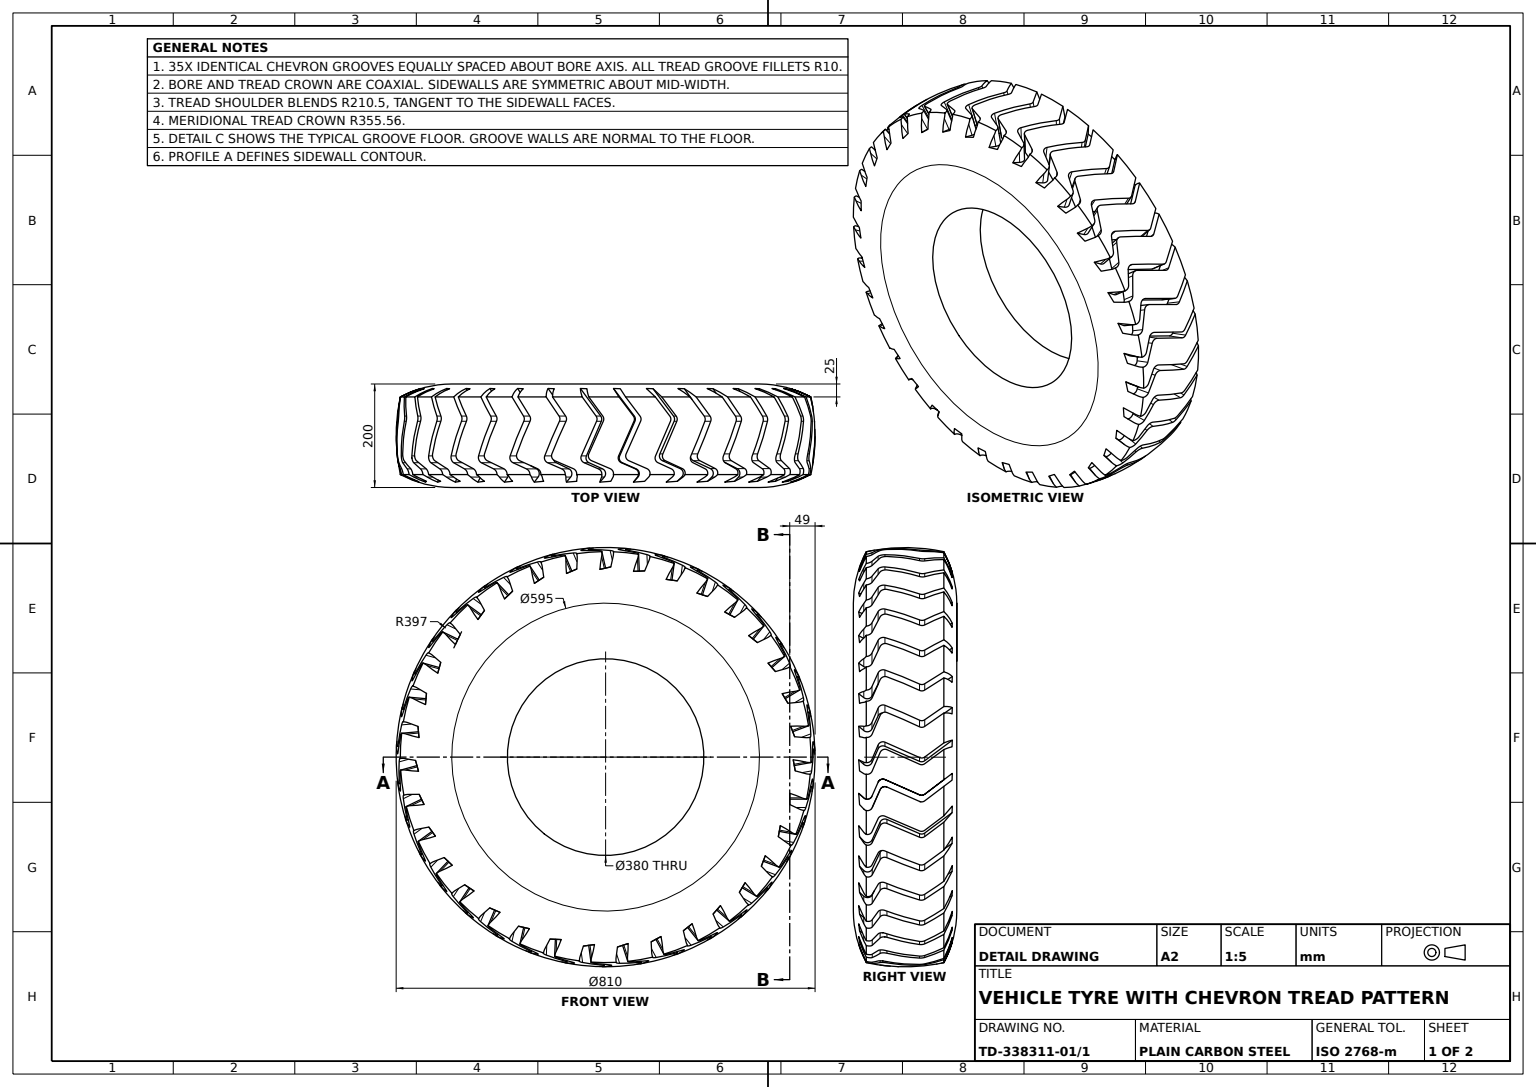
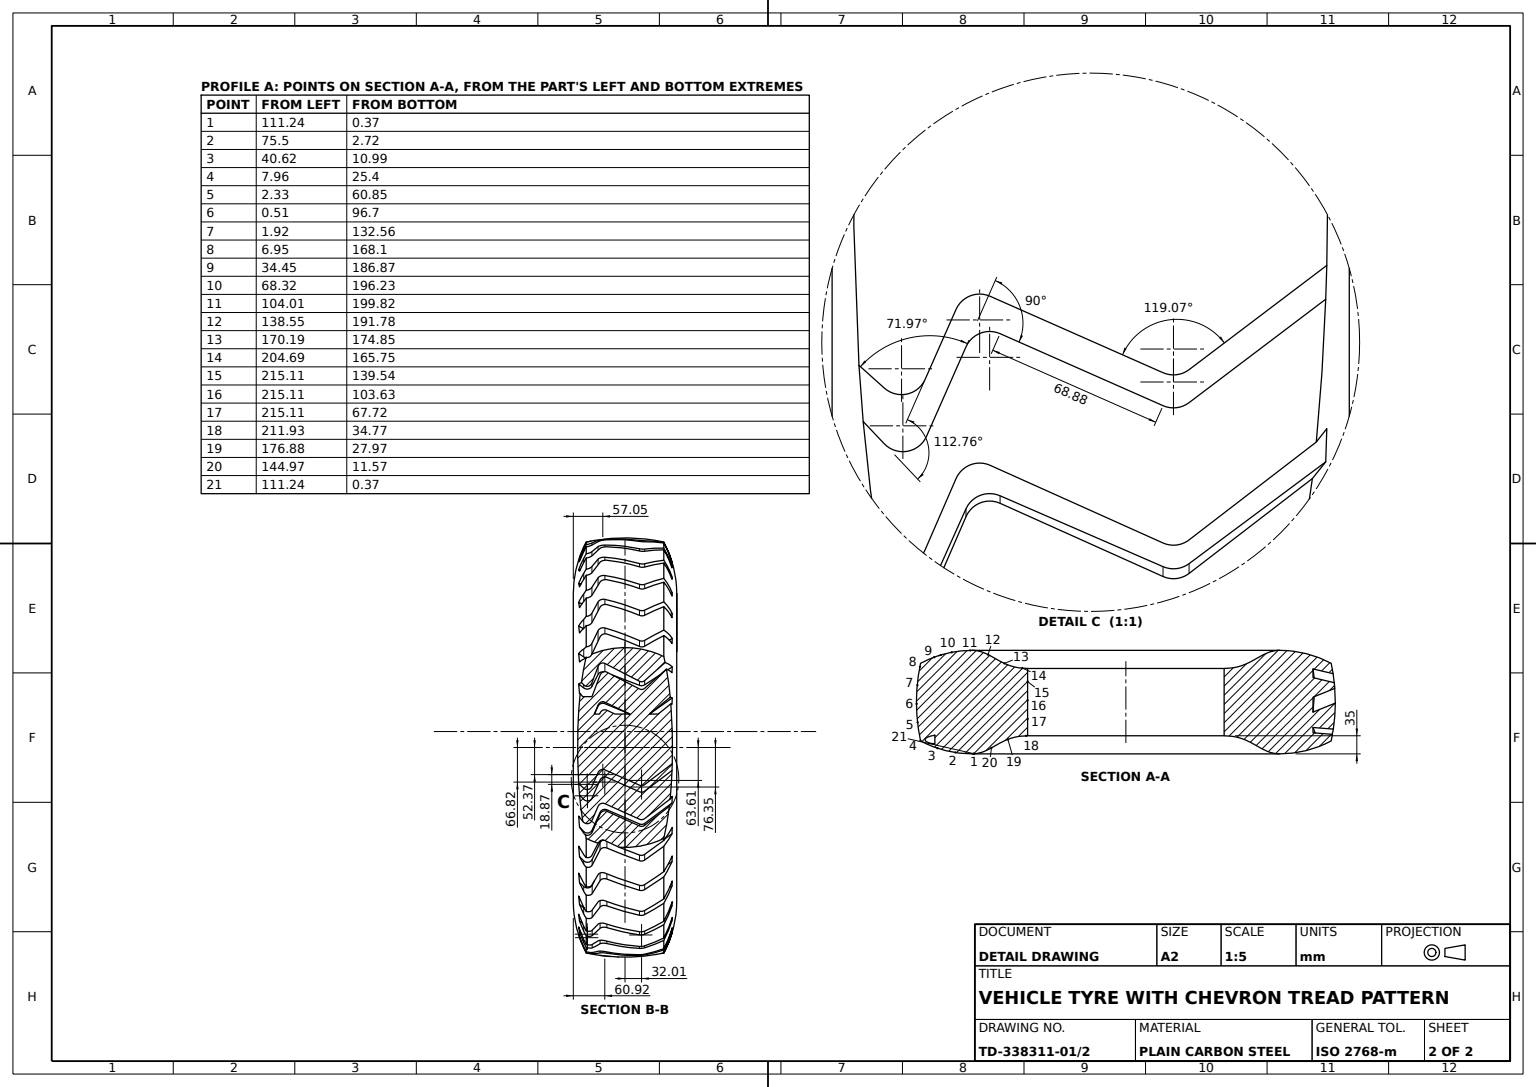
SolidWorks part; units mm, degrees
material "Plain Carbon Steel"
ref_plane "Front Plane" through (0, 0, 0) normal (0, 0, 1) x (1, 0, 0)
ref_plane "Top Plane" through (0, 0, 0) normal (0, 1, 0) x (1, 0, 0)
ref_plane "Right Plane" through (0, 0, 0) normal (1, 0, 0) x (0, 0, -1)
sketch "Tyre Section Profile" plane through (0, 0, 0) normal (0, 0, 1) x (1, 0, 0)
  line L0 (0, 0) -> (399.8598, 0) construction
  line L1 (0, 297.5) -> (0, 538.6574) construction
  line L2 (-100, 405) -> (100, 405)
  line L3 (-100, 405) -> (-100, 190)
  line L4 (-100, 190) -> (100, 190)
  line L5 (100, 405) -> (100, 190)
  line L6 (-100, 405) -> (100, 190) construction
  line L7 (-100, 190) -> (100, 405) construction
  line L8 (-65, 146.7783) -> (-65, 233.2217) construction
  line L9 (-45, 190) -> (65, 190)
  arc A0 (-75, 397) -> (75, 397) centre (0, 49.4375) cw
  arc A1 (-75, 397) -> (-100, 297.5) centre (110.505, 297.5) ccw
  arc A2 (75, 397) -> (100, 297.5) centre (-110.505, 297.5) cw
  arc A3 (-65, 190) -> (-45, 190) centre (-55, 190) ccw
  spline S0 degree 3 poles (-100, 297.5) (-100, 259.1667) (-65, 244.0271) (-65, 190) knots 0 0 0 0 1 1 1 1
  spline S1 degree 3 poles (100, 297.5) (100, 259.1667) (65, 244.0271) (65, 190) knots 0 0 0 0 1 1 1 1
  point P3 (0, 297.5)
  point P9 (-75, 397)
  point P11 (75, 397)
  point P17 (-65, 190)
  dimension "D6" = 35
  dimension "D7" = 115
  dimension "D8" = 210.505
  dimension "D9" = 10
  dimension "D1" = 215
  dimension "D2" = 200
  dimension "D3" = 190
  dimension "D4" = 8
  dimension "D5" = 25
revolve "Tyre Body" add sketch "Tyre Section Profile" angle 360 about L0
sketch "Tread Boundary Profile" plane through (0, 0, 0) normal (0, 0, 1) x (1, 0, 0)
  line L0 (-123.917, 370) -> (-90.3548, 370)
  line L1 (-75, 397) -> (-75, -397) construction
  line L2 (-75, 375.5015) -> (-38.1785, 381.9941)
  line L3 (-20, 400) -> (28.0546, 400)
  line L4 (0, 0) -> (0, 545.0765) construction
  line L5 (0, 0) -> (475.9247, 0) construction
  line L6 (123.917, 370) -> (90.3548, 370)
  line L7 (75, 375.5015) -> (38.1785, 381.9941)
  arc A0 (38.1785, 381.9941) -> (29.9575, 390.9211) centre (39.915, 391.8422) cw
  arc A1 (-38.1785, 381.9941) -> (-29.9575, 390.9211) centre (-39.915, 391.8422) ccw
  arc A2 (-29.9575, 390.9211) -> (-20, 400) centre (-20, 390) cw
  arc A3 (29.9575, 390.9211) -> (20, 400) centre (20, 390) ccw
  spline S0 degree 3 poles (-75, 375.5015) (-80.894, 374.4622) (-84.1463, 370) (-90.3548, 370) knots 0 0 0 0 1 1 1 1
  spline S1 degree 3 poles (75, 375.5015) (80.894, 374.4622) (84.1463, 370) (90.3548, 370) knots 0 0 0 0 1 1 1 1
  dimension "D1" = 10
  dimension "D2" = 10
  dimension "D3" = 20
  dimension "D4" = 170
  dimension "D5" = 30
  dimension "D6" = 400
  dimension "D7" = 28.0546
  dimension "D8" = 29.9575
  dimension "D9" = 90.3548
  dimension "D10" = 123.917
surface "Tread Boundary Surface" sketch "Tread Boundary Profile" parameters "D1"=360
ref_plane "Tread Sketch Plane" through (0, 410, 0) normal (0, 1, 0) x (1, 0, 0)
sketch "Tread Groove Sketch" plane through (0, 410, 0) normal (0, 1, 0) x (1, 0, 0)
  line L0 (-123.917, 19.3848) -> (-38.0439, 84.3298)
  line L1 (-123.917, -370) -> (-123.917, 370) construction
  line L2 (-27.9717, 85.5015) -> (35.0394, 57.6715)
  line L3 (48.2271, 62.7789) -> (63.4843, 97.3234)
  line L4 (79.8956, 100.1562) -> (123.917, 53.6314)
  line L5 (123.917, -370) -> (123.917, 370) construction
  line L6 (123.917, 53.6314) -> (123.917, 39.183)
  line L7 (123.917, 39.183) -> (79.8165, 78.6897)
  line L8 (63.9965, 75.2815) -> (52.0932, 48.3305)
  line L9 (38.9055, 43.2231) -> (-27.9717, 72.7606)
  line L10 (-38.0439, 71.5889) -> (-123.917, 6.6439)
  line L11 (-123.917, 6.6439) -> (-123.917, 19.3848)
  arc A0 (35.0394, 57.6715) -> (48.2271, 62.7789) centre (39.0796, 66.8191) ccw
  arc A1 (52.0932, 48.3305) -> (38.9055, 43.2231) centre (42.9456, 52.3707) cw
  arc A2 (79.8165, 78.6897) -> (63.9965, 75.2815) centre (73.144, 71.2414) ccw
  arc A3 (63.4843, 97.3234) -> (79.8956, 100.1562) centre (72.6318, 93.2833) cw
  arc A4 (-27.9717, 72.7606) -> (-38.0439, 71.5889) centre (-32.0119, 63.613) ccw
  arc A5 (-38.0439, 84.3298) -> (-27.9717, 85.5015) centre (-32.0119, 76.3539) cw
  dimension "D1" = 10
  dimension "D2" = 32.0119
  dimension "D3" = 76.3539
  dimension "D4" = 10.162
  dimension "D5" = 19.3848
  dimension "D6" = 119.071
  dimension "D7" = 68.8833
  dimension "D8" = 9.3738
  dimension "D9" = 37.7638
  dimension "D10" = 29.4627
  dimension "D11" = 53.6314
  dimension "D12" = 39.183
extrude "Tread Groove Cut" cut sketch "Tread Groove Sketch" against normal blind 54
pattern_circular "Tread Groove Pattern 35x" count 35 over 360 about axis through (0, 0, 0) along (1, 0, 0) of "Tread Groove Cut"
delete or keep bodies "Body-Delete/Keep 1" type delete bodies bodies 102 103
